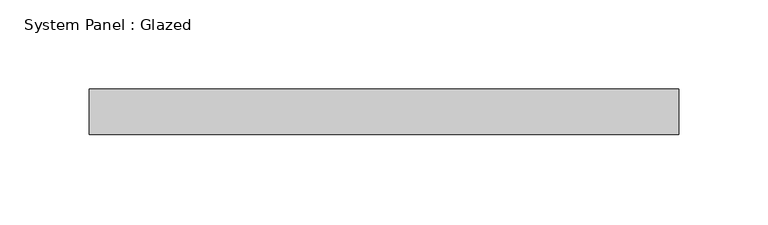
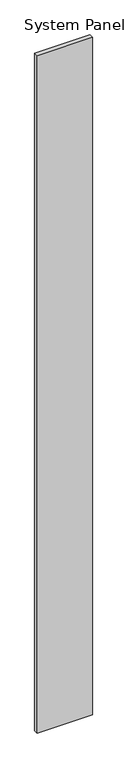
"""IFC4 building model written with IfcOpenShell, lengths in millimetres: plate geometry, System Panel : Glazed."""

from ifc_helpers import new_model, si_unit, origin, origin_with_axes, place, context, project, spatial, polyline, outline, extrude, source, transform, mapped, element, save


def system_panel_glazed_5fe90612(model_context):
    return source(origin(), model_context, "Body", "SweptSolid", [
        extrude(outline(polyline([(165.1, 19.05), (-165.1, 19.05), (-165.1, 44.45), (165.1, 44.45), (165.1, 19.05)])), origin_with_axes(), (0.0, 0.0, 1.0), 4288.4575854),
    ])


if __name__ == "__main__":
    model = new_model("IFC4")
    model_context = context("Model", 3, world=origin())
    ifc_project = project(units=[si_unit("LENGTHUNIT", "METRE", prefix="MILLI")], contexts=[model_context])
    site = spatial("IfcSite", under=ifc_project)
    building = spatial("IfcBuilding", under=site)
    placement = place(None, origin())
    system_panel_glazed_shape = system_panel_glazed_5fe90612(model_context)
    element("IfcPlate", 1, ObjectType="System Panel : Glazed", at=placement, inside=building, context=model_context, shape_type="MappedRepresentation", body=[
        mapped(system_panel_glazed_shape, transform((0.0, 0.0, 0.0), x_axis=(1.0, 0.0, 0.0), y_axis=(0.0, 1.0, 0.0), z_axis=(0.0, 0.0, 1.0))),
    ])
    save(model, "model.ifc")

# Revit data of these elements
# Type "System Panel : Glazed"
#   Construction Type Id = "GSP4R"
#   Analytic Construction = "1/8 in Pilkington single glazing"
#   Visual Light Transmittance = 0.9
#   Solar Heat Gain Coefficient = 0.86
#   Heat Transfer Coefficient (U) = 1.18115 BTU/(h·ft²·°F)
#   Define Thermal Properties by = 1
# Element 1 (IfcPlate, "System Panel : Glazed")
#   Materials on its faces: "Glass"
# Materials
#   "Glass": class "Glass", colour RGB 0 128 192, transparency 0.75, Description = "Soda Lime Glass", Cost = 0
